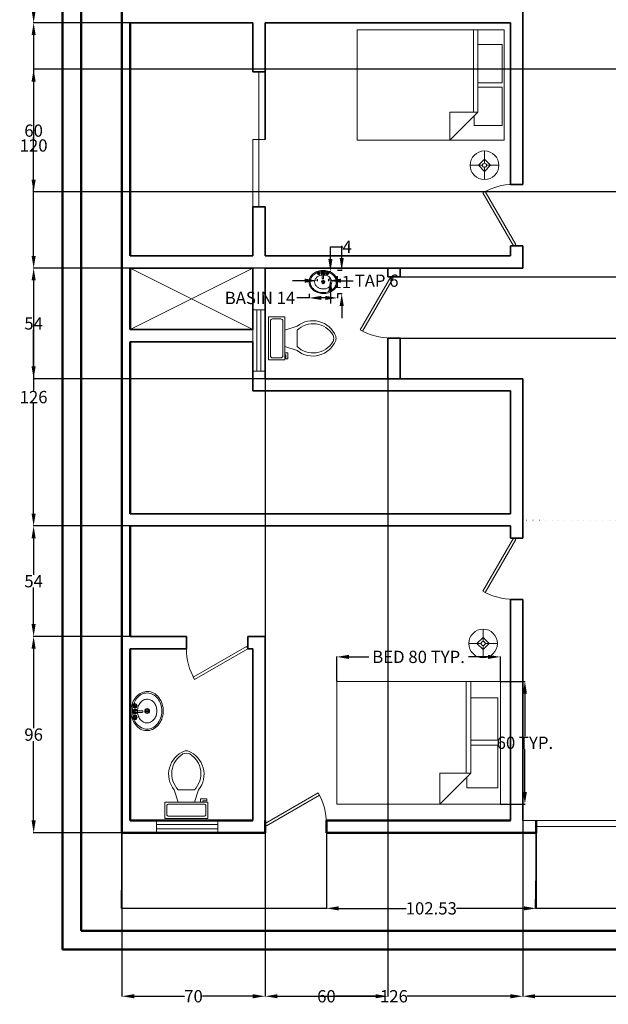
# Model space of a CAD drawing. Units: inches. Extents: x 910 to 1553, y 598 to 1516.
# Tile 1 of 6: x 910 to 1198, y 598 to 1079. Entities that reach past the tile are written whole.
import ezdxf

# ---------------------------------------------------------------- set-up
doc = ezdxf.new("R2010")
doc.units = ezdxf.units.IN
doc.header["$MEASUREMENT"] = 0
doc.linetypes.add('ACAD_ISO07W100', pattern=[3, 0, -3])
for name, color, linetype, lineweight in [('A-ANNO-DIMS', 2, 'Continuous', 18), ('A-FLOR-BALC', 8, 'Continuous', 25), ('A-FLOR-OPEN', 8, 'Continuous', 13), ('A-FLOR-OVHD', 8, 'ACAD_ISO07W100', 13), ('doors', 2, 'Continuous', 18), ('furniture', 11, 'Continuous', 18), ('Inner wall', 230, 'Continuous', 35), ('outer wall', 231, 'Continuous', 50), ('sanitory', 141, 'Continuous', 18), ('windows', 6, 'Continuous', 18)]:
    doc.layers.add(name, color=color, linetype=linetype, lineweight=lineweight)
doc.styles.get("Standard").update_dxf_attribs({"font": 'arial.ttf'})
doc.dimstyles.get("Standard").update_dxf_attribs({"dimtxt": 6, "dimasz": 6, "dimexe": 0.18, "dimexo": 0.0625, "dimgap": 0.09, "dimtad": 0, "dimtih": 1, "dimtoh": 1, "dimdec": 0, "dimzin": 0, "dimdsep": 46, "dimlunit": 3, "dimtxsty": 'Standard', "dimcen": 0.09, "dimadec": 0, "dimazin": 0, "dimtfac": 1, "dimtdec": 0, "dimtofl": 0, "dimtmove": 0, "dimatfit": 3, "dimfxl": 1, "dimtolj": 1, "dimtzin": 0, "dimarcsym": 0})

# ---------------------------------------------------------------- blocks, each defined once
blk = doc.blocks.new('*U7')
for p, q in [((-40, 0), (-40, 6)), ((0, 0), (0, 6))]:
    blk.add_line(p, q)
blk.add_lwpolyline([(0, 0), (-34.64, -20), (-35.52, -18.48), (-0.88, 1.52)], close=True)
blk.add_arc((0, 0), 40, 180, 210)
blk = doc.blocks.new('*U2')
for p, q in [((0, 0), (0, -6)), ((40, 0), (40, -6))]:
    blk.add_line(p, q)
blk.add_lwpolyline([(0, 0), (34.64, 20), (35.52, 18.48), (0.87, -1.52)], close=True)
blk.add_arc((0, 0), 40, 0, 30)
blk = doc.blocks.new('*U5')
for p, q in [((0, 0), (0, -6)), ((-40, 0), (-40, -6))]:
    blk.add_line(p, q)
blk.add_lwpolyline([(0, 0), (-34.64, 20), (-35.52, 18.48), (-0.88, -1.52)], close=True)
blk.add_arc((0, 0), 40, 150, 180)
blk = doc.blocks.new('Toilet - top')
for p, q in [((9.5, -6), (9.5, -2)), ((-10, -8.5), (-8, -8.5)), ((-10, -9.5), (-10, -8.5)), ((-7, -9.5), (-10, -9.5)), ((-8, -8.5), (-8, -8)), ((-7, -8), (-7, -9.5)), ((-4, -8), (-6, -14)), ((4, -8), (6, -14)), ((4, -14), (-4, -14))]:
    blk.add_line(p, q)
blk.add_lwpolyline([(10.5, -8), (10.5, 0), (-10.5, 0), (-10.5, -8)], close=True)
for points in [[(-9.5, -2), (-9.5, -6)], [(8.5, -1), (-8.5, -1)], [(-8.5, -7), (8.5, -7)]]:
    blk.add_lwpolyline(points)
for centre, radius, start, end in [((-8.62, -1.88), 0.884, 81.8699, 188.1301), ((8.62, -1.88), 0.884, 351.8699, 98.1301), ((-8.62, -6.12), 0.884, 171.8699, 278.1301), ((8.62, -6.12), 0.884, 261.8699, 8.1301), ((3.52, -21.58), 12.17, 141.4691, 247.9714), ((4.2, -21.82), 11.33, 136.3677, 238.9468), ((-3.52, -21.58), 12.17, 292.0284, 38.5307), ((-4.2, -21.82), 11.33, 301.053, 43.6321), ((0, -27.88), 4, 245.7318, 294.2682), ((0, -29), 4, 254.8605, 285.1395)]:
    blk.add_arc(centre, radius, start, end)
blk = doc.blocks.new('Bed - Queen')
for p, q in [((0, -80.00003), (0, 0)), ((0, 0), (59.99999, 0)), ((59.99999, 0), (59.99999, -80.00003)), ((7.99999, -1.2), (28.79998, -1.2)), ((7.99999, -14.4), (7.99999, -1.2)), ((28.79998, -1.2), (28.79998, -14.4)), ((31.19999, -1.2), (51.99999, -1.2)), ((31.19999, -14.4), (31.19999, -1.2)), ((51.99999, -1.2), (51.99999, -16.4)), ((0, -14.4), (44.8, -14.4)), ((59.99999, -29.6), (44.8, -14.4)), ((44.8, -14.4), (44.8, -29.6)), ((44.8, -16.8), (0, -16.8)), ((51.99999, -16.4), (46.79936, -16.4)), ((44.8, -29.6), (59.99999, -29.6)), ((59.99999, -80.00003), (0, -80.00003))]:
    blk.add_line(p, q)
blk = doc.blocks.new('Lamp - Table')
for p, q in [((0, 7), (0, 1)), ((-1, 0), (-7, 0)), ((0, 3), (-3, 0)), ((-3, 0), (0, -3)), ((3, 0), (0, 3)), ((0, -3), (3, 0)), ((1, 0), (7, 0)), ((0, -1), (0, -7))]:
    blk.add_line(p, q)
for radius in [7, 1]:
    blk.add_circle((0, 0), radius)
blk = doc.blocks.new('Faucet - Bathroom top')
for p, q in [((-4.107, 0.125), (-4.375, 0.125)), ((-3.75, 0.4788), (-3.75, 0.75)), ((-3.5, 0.482), (-3.5, 0.75)), ((-3.1461, 0.125), (-2.875, 0.125)), ((3.143, 0.125), (2.875, 0.125)), ((3.5, 0.4788), (3.5, 0.75)), ((3.75, 0.482), (3.75, 0.75)), ((4.1039, 0.125), (4.375, 0.125)), ((-4.1039, -0.125), (-4.375, -0.125)), ((-3.75, -0.4821), (-3.75, -0.75)), ((-3.5, -0.4789), (-3.5, -0.75)), ((-3.143, -0.125), (-2.875, -0.125)), ((-0.5, -0.8639), (-0.5, -4.5)), ((0.5, -4.5), (0.5, -0.8631)), ((3.1461, -0.125), (2.875, -0.125)), ((3.5, -0.4821), (3.5, -0.75)), ((3.75, -0.4789), (3.75, -0.75)), ((4.107, -0.125), (4.375, -0.125))]:
    blk.add_line(p, q)
for centre, radius in [((-3.625, 0), 1.375), ((-4.625, 0), 0.2795), ((-3.625, 0), 0.5), ((-3.625, 1), 0.2795), ((-2.625, 0), 0.2795), ((0, 0), 0.5), ((3.625, 0), 1.375), ((2.625, 0), 0.2795), ((3.625, 0), 0.5), ((3.625, 1), 0.2795), ((4.625, 0), 0.2795), ((-3.625, -1), 0.2795), ((3.625, -1), 0.2795)]:
    blk.add_circle(centre, radius)
for centre, radius, start, end in [((-3.625, 0), 1, 105.2407, 164.2093), ((-3.625, 0), 1, 16.44125, 74.07887), ((0, 0), 1.5, 289.6514, 250.3603), ((0, 0), 1, 300.3431, 239.7554), ((3.625, 0), 1, 106.12, 164.0884), ((3.625, 0), 1, 16.23422, 73.90469), ((-3.625, 0), 1, 196.2342, 253.9047), ((-3.625, 0), 1, 286.12, 344.0884), ((0, -4.5), 0.5, 180, 0), ((3.625, 0), 1, 196.4413, 254.0789), ((3.625, 0), 1, 285.2407, 344.2093)]:
    blk.add_arc(centre, radius, start, end)
blk = doc.blocks.new('Sink - Oval top')
for p, q in [((-1, 0), (1, 0)), ((0, 1), (0, -1))]:
    blk.add_line(p, q)
for points in [[(-12.23, 0.39, 0.117634), (-11.46, -3.36, 0.104469), (-8.88, -6.8, 0.090016), (-5.08, -9.07, 0.08192), (-0.32, -10.02, 0.08192), (4.49, -9.38, 0.090016), (8.42, -7.36, 0.104469), (11.22, -4.09, 0.117634), (12.23, -0.39, 0.117634), (11.46, 3.36, 0.104469), (8.88, 6.8, 0.090016), (5.08, 9.07, 0.08192), (0.32, 10.02, 0.08192), (-4.49, 9.38, 0.090016), (-8.42, 7.36, 0.104469), (-11.22, 4.09, 0.117634)], [(-11.29, 0.16, 0.118622), (-10.52, -3.25, 0.104678), (-8.07, -6.36, 0.089562), (-4.54, -8.37, 0.081185), (-0.13, -9.15, 0.081185), (4.3, -8.49, 0.089562), (7.89, -6.58, 0.104678), (10.42, -3.55, 0.118622), (11.29, -0.16, 0.118622), (10.52, 3.25, 0.104678), (8.07, 6.36, 0.089562), (4.54, 8.37, 0.081185), (0.13, 9.15, 0.081185), (-4.3, 8.49, 0.089562), (-7.89, 6.58, 0.104678), (-10.42, 3.55, 0.118622)], [(-7.42, 0.08, 0.118283), (-6.91, -2.17, 0.104607), (-5.29, -4.21, 0.089718), (-2.97, -5.53, 0.081436), (-0.07, -6.04, 0.081436), (2.84, -5.59, 0.089718), (5.2, -4.33, 0.104607), (6.86, -2.32, 0.118283), (7.42, -0.08, 0.118283), (6.91, 2.17, 0.104607), (5.29, 4.21, 0.089718), (2.97, 5.53, 0.081436), (0.07, 6.04, 0.081436), (-2.84, 5.59, 0.089718), (-5.2, 4.33, 0.104607), (-6.86, 2.32, 0.118283)]]:
    blk.add_lwpolyline(points, format="xyb", close=True)
for radius in [1.5, 1]:
    blk.add_circle((0, 0), radius)
blk = doc.blocks.new('WIN-30X6')
for p, q in [((0, 6), (30, 6)), ((0, 0), (0, 6)), ((30, 6), (30, 0)), ((0, 4), (30, 4)), ((30, 2), (0, 2)), ((30, 0), (0, 0))]:
    blk.add_line(p, q)
blk = doc.blocks.new('VERANDA-EDGE-DEEP')
for p, q in [((0.23, 17.99), (0.23, 36.98)), ((100.23, 36.98), (100.23, 17.99)), ((0, 0), (0.23, 17.99)), ((100.23, 17.99), (100.23, 0)), ((100.23, 0), (0, 0))]:
    blk.add_line(p, q)
blk = doc.blocks.new('*D25')
at = {"layer": 'A-ANNO-DIMS', "color": 0, "lineweight": -2, "transparency": 16777216}
for p, q in [((1064.74, 756.03), (1064.74, 768.14)), ((1070.74, 767.96), (1080.4, 767.96)), ((1138.74, 767.96), (1129.09, 767.96)), ((1144.74, 756.03), (1144.74, 768.14))]:
    blk.add_line(p, q, dxfattribs=at)
for points in [[(1070.74, 768.96), (1070.74, 766.96), (1064.74, 767.96)], [(1138.74, 768.96), (1138.74, 766.96), (1144.74, 767.96)]]:
    blk.add_solid(points, dxfattribs=at)
at = {"layer": 'Defpoints', "color": 0, "lineweight": -2, "transparency": 16777216}
for p in [(1144.74, 767.96), (1064.74, 755.96), (1144.74, 755.96)]:
    blk.add_point(p, dxfattribs=at)
at = {"layer": 'A-ANNO-DIMS', "color": 0, "transparency": 16777216, "insert": (1104.74, 767.96), "char_height": 6, "attachment_point": 5}
blk.add_mtext('\\A1;BED 80 TYP.', dxfattribs=at)
blk = doc.blocks.new('*D26')
at = {"layer": 'A-ANNO-DIMS', "color": 0, "lineweight": -2, "transparency": 16777216}
for p, q in [((1144.81, 755.96), (1156.92, 755.96)), ((1156.74, 749.96), (1156.74, 729.12)), ((1156.74, 701.96), (1156.74, 722.81)), ((1144.81, 695.96), (1156.92, 695.96))]:
    blk.add_line(p, q, dxfattribs=at)
for points in [[(1155.74, 749.96), (1157.74, 749.96), (1156.74, 755.96)], [(1155.74, 701.96), (1157.74, 701.96), (1156.74, 695.96)]]:
    blk.add_solid(points, dxfattribs=at)
at = {"layer": 'Defpoints', "color": 0, "lineweight": -2, "transparency": 16777216}
for p in [(1144.74, 755.96), (1144.74, 695.96), (1156.74, 695.96)]:
    blk.add_point(p, dxfattribs=at)
at = {"layer": 'A-ANNO-DIMS', "color": 0, "transparency": 16777216, "insert": (1156.74, 725.96), "char_height": 6, "attachment_point": 5}
blk.add_mtext('\\A1;60 TYP.', dxfattribs=at)
blk = doc.blocks.new('*D33')
at = {"layer": 'A-ANNO-DIMS', "color": 0, "lineweight": -2, "transparency": 16777216}
for p, q in [((1051.19, 945.48), (1051.19, 943.27)), ((1065.09, 945.48), (1065.09, 943.27)), ((1051.19, 943.45), (1045.19, 943.45)), ((1059.09, 943.45), (1057.19, 943.45))]:
    blk.add_line(p, q, dxfattribs=at)
for points in [[(1057.19, 944.45), (1057.19, 942.45), (1051.19, 943.45)], [(1059.09, 944.45), (1059.09, 942.45), (1065.09, 943.45)]]:
    blk.add_solid(points, dxfattribs=at)
at = {"layer": 'Defpoints', "color": 0, "lineweight": -2, "transparency": 16777216}
for p in [(1051.19, 945.54), (1065.09, 945.54), (1051.19, 943.45)]:
    blk.add_point(p, dxfattribs=at)
at = {"layer": 'A-ANNO-DIMS', "color": 0, "transparency": 16777216, "insert": (1027.2, 943.45), "char_height": 6, "attachment_point": 5}
blk.add_mtext('\\A1;BASIN 14', dxfattribs=at)
blk = doc.blocks.new('*D34')
at = {"layer": 'A-ANNO-DIMS', "color": 0, "lineweight": -2, "transparency": 16777216}
for p, q in [((1067.17, 962.94), (1067.17, 968.94)), ((1065.15, 956.94), (1067.35, 956.94)), ((1065.15, 945.54), (1067.35, 945.54)), ((1067.17, 939.54), (1067.17, 933.54))]:
    blk.add_line(p, q, dxfattribs=at)
for points in [[(1066.17, 962.94), (1068.17, 962.94), (1067.17, 956.94)], [(1066.17, 939.54), (1068.17, 939.54), (1067.17, 945.54)]]:
    blk.add_solid(points, dxfattribs=at)
at = {"layer": 'Defpoints', "color": 0, "lineweight": -2, "transparency": 16777216}
for p in [(1065.09, 956.94), (1065.09, 945.54), (1067.17, 945.54)]:
    blk.add_point(p, dxfattribs=at)
at = {"layer": 'A-ANNO-DIMS', "color": 0, "transparency": 16777216, "insert": (1067.17, 951.24), "char_height": 6, "attachment_point": 5}
blk.add_mtext('\\A1;11', dxfattribs=at)
blk = doc.blocks.new('*D37')
at = {"layer": 'A-ANNO-DIMS', "color": 0, "lineweight": -2, "transparency": 16777216}
for p, q in [((1049.13, 951.87), (1043.13, 951.87)), ((1055.13, 952.66), (1055.13, 951.69)), ((1060.79, 952.66), (1060.79, 951.69)), ((1066.79, 951.87), (1072.79, 951.87))]:
    blk.add_line(p, q, dxfattribs=at)
for points in [[(1049.13, 952.87), (1049.13, 950.87), (1055.13, 951.87)], [(1066.79, 952.87), (1066.79, 950.87), (1060.79, 951.87)]]:
    blk.add_solid(points, dxfattribs=at)
at = {"layer": 'Defpoints', "color": 0, "lineweight": -2, "transparency": 16777216}
for p in [(1055.13, 952.72), (1060.79, 952.72), (1060.79, 951.87)]:
    blk.add_point(p, dxfattribs=at)
at = {"layer": 'A-ANNO-DIMS', "color": 0, "transparency": 16777216, "insert": (1084.24, 951.87), "char_height": 6, "attachment_point": 5}
blk.add_mtext('\\A1;TAP 6', dxfattribs=at)
blk = doc.blocks.new('*D38')
at = {"layer": 'A-ANNO-DIMS', "color": 0, "lineweight": -2, "transparency": 16777216}
for p, q in [((1061.64, 962.4), (1061.64, 968.4)), ((1061.64, 968.4), (1067.64, 968.4)), ((1060.85, 956.4), (1061.82, 956.4)), ((1060.85, 952.72), (1061.82, 952.72)), ((1061.64, 946.72), (1061.64, 940.72))]:
    blk.add_line(p, q, dxfattribs=at)
for points in [[(1060.64, 962.4), (1062.64, 962.4), (1061.64, 956.4)], [(1060.64, 946.72), (1062.64, 946.72), (1061.64, 952.72)]]:
    blk.add_solid(points, dxfattribs=at)
at = {"layer": 'Defpoints', "color": 0, "lineweight": -2, "transparency": 16777216}
for p in [(1060.79, 956.4), (1061.64, 956.4), (1060.79, 952.72)]:
    blk.add_point(p, dxfattribs=at)
at = {"layer": 'A-ANNO-DIMS', "color": 0, "transparency": 16777216, "insert": (1069.81, 968.4), "char_height": 6, "attachment_point": 5}
blk.add_mtext('\\A1;4', dxfattribs=at)
blk = doc.blocks.new('*D57')
at = {"layer": 'A-ANNO-DIMS', "color": 0, "lineweight": -2, "transparency": 16777216}
for p, q in [((959.7, 681.91), (959.7, 601.86)), ((1029.7, 681.91), (1029.7, 601.86)), ((965.7, 602.04), (990.35, 602.04)), ((1023.7, 602.04), (999.05, 602.04))]:
    blk.add_line(p, q, dxfattribs=at)
for points in [[(965.7, 603.04), (965.7, 601.04), (959.7, 602.04)], [(1023.7, 603.04), (1023.7, 601.04), (1029.7, 602.04)]]:
    blk.add_solid(points, dxfattribs=at)
at = {"layer": 'Defpoints', "color": 0, "lineweight": -2, "transparency": 16777216}
for p in [(959.7, 681.97), (1029.7, 681.97), (1029.7, 602.04)]:
    blk.add_point(p, dxfattribs=at)
at = {"layer": 'A-ANNO-DIMS', "color": 0, "transparency": 16777216, "insert": (994.7, 602.04), "char_height": 6, "attachment_point": 5}
blk.add_mtext('\\A1;70', dxfattribs=at)
blk = doc.blocks.new('*D58')
at = {"layer": 'A-ANNO-DIMS', "color": 0, "lineweight": -2, "transparency": 16777216}
for p, q in [((1155.7, 687.91), (1155.7, 601.86)), ((1029.7, 681.91), (1029.7, 601.86)), ((1035.7, 602.04), (1086.27, 602.04)), ((1149.7, 602.04), (1099.13, 602.04))]:
    blk.add_line(p, q, dxfattribs=at)
for points in [[(1035.7, 603.04), (1035.7, 601.04), (1029.7, 602.04)], [(1149.7, 603.04), (1149.7, 601.04), (1155.7, 602.04)]]:
    blk.add_solid(points, dxfattribs=at)
at = {"layer": 'Defpoints', "color": 0, "lineweight": -2, "transparency": 16777216}
for p in [(1155.7, 687.97), (1029.7, 681.97), (1155.7, 602.04)]:
    blk.add_point(p, dxfattribs=at)
at = {"layer": 'A-ANNO-DIMS', "color": 0, "transparency": 16777216, "insert": (1092.7, 602.04), "char_height": 6, "attachment_point": 5}
blk.add_mtext('\\A1;126', dxfattribs=at)
blk = doc.blocks.new('*D59')
at = {"layer": 'A-ANNO-DIMS', "color": 0, "lineweight": -2, "transparency": 16777216}
for p, q in [((1155.7, 687.91), (1155.7, 601.86)), ((1281.7, 687.91), (1281.7, 601.86)), ((1161.7, 602.04), (1212.27, 602.04)), ((1275.7, 602.04), (1225.13, 602.04))]:
    blk.add_line(p, q, dxfattribs=at)
for points in [[(1161.7, 603.04), (1161.7, 601.04), (1155.7, 602.04)], [(1275.7, 603.04), (1275.7, 601.04), (1281.7, 602.04)]]:
    blk.add_solid(points, dxfattribs=at)
at = {"layer": 'Defpoints', "color": 0, "lineweight": -2, "transparency": 16777216}
for p in [(1155.7, 687.97), (1281.7, 687.97), (1281.7, 602.04)]:
    blk.add_point(p, dxfattribs=at)
at = {"layer": 'A-ANNO-DIMS', "color": 0, "transparency": 16777216, "insert": (1218.7, 602.04), "char_height": 6, "attachment_point": 5}
blk.add_mtext('\\A1;126', dxfattribs=at)
blk = doc.blocks.new('*D62')
at = {"layer": 'A-ANNO-DIMS', "color": 0, "lineweight": -2, "transparency": 16777216}
for p, q in [((963.64, 777.97), (916.34, 777.97)), ((916.52, 771.97), (916.52, 733.12)), ((916.52, 687.97), (916.52, 726.82)), ((959.64, 681.97), (916.34, 681.97))]:
    blk.add_line(p, q, dxfattribs=at)
for points in [[(915.52, 771.97), (917.52, 771.97), (916.52, 777.97)], [(915.52, 687.97), (917.52, 687.97), (916.52, 681.97)]]:
    blk.add_solid(points, dxfattribs=at)
at = {"layer": 'Defpoints', "color": 0, "lineweight": -2, "transparency": 16777216}
for p in [(916.52, 777.97), (963.7, 777.97), (959.7, 681.97)]:
    blk.add_point(p, dxfattribs=at)
at = {"layer": 'A-ANNO-DIMS', "color": 0, "transparency": 16777216, "insert": (916.52, 729.97), "char_height": 6, "attachment_point": 5}
blk.add_mtext('\\A1;96', dxfattribs=at)
blk = doc.blocks.new('*D63')
at = {"layer": 'A-ANNO-DIMS', "color": 0, "lineweight": -2, "transparency": 16777216}
for p, q in [((963.64, 831.97), (916.34, 831.97)), ((916.52, 825.97), (916.52, 808.11)), ((916.52, 783.97), (916.52, 801.83)), ((963.64, 777.97), (916.34, 777.97))]:
    blk.add_line(p, q, dxfattribs=at)
for points in [[(915.52, 825.97), (917.52, 825.97), (916.52, 831.97)], [(915.52, 783.97), (917.52, 783.97), (916.52, 777.97)]]:
    blk.add_solid(points, dxfattribs=at)
at = {"layer": 'Defpoints', "color": 0, "lineweight": -2, "transparency": 16777216}
for p in [(916.52, 831.97), (963.7, 831.97), (963.7, 777.97)]:
    blk.add_point(p, dxfattribs=at)
at = {"layer": 'A-ANNO-DIMS', "color": 0, "transparency": 16777216, "insert": (916.52, 804.97), "char_height": 6, "attachment_point": 5}
blk.add_mtext('\\A1;54', dxfattribs=at)
blk = doc.blocks.new('*D64')
at = {"layer": 'A-ANNO-DIMS', "color": 0, "lineweight": -2, "transparency": 16777216}
for p, q in [((963.64, 957.97), (916.34, 957.97)), ((916.52, 951.97), (916.52, 898.12)), ((916.52, 837.97), (916.52, 891.82)), ((963.64, 831.97), (916.34, 831.97))]:
    blk.add_line(p, q, dxfattribs=at)
for points in [[(915.52, 951.97), (917.52, 951.97), (916.52, 957.97)], [(915.52, 837.97), (917.52, 837.97), (916.52, 831.97)]]:
    blk.add_solid(points, dxfattribs=at)
at = {"layer": 'Defpoints', "color": 0, "lineweight": -2, "transparency": 16777216}
for p in [(916.52, 957.97), (963.7, 957.97), (963.7, 831.97)]:
    blk.add_point(p, dxfattribs=at)
at = {"layer": 'A-ANNO-DIMS', "color": 0, "transparency": 16777216, "insert": (916.52, 894.97), "char_height": 6, "attachment_point": 5}
blk.add_mtext('\\A1;126', dxfattribs=at)
blk = doc.blocks.new('*D65')
at = {"layer": 'A-ANNO-DIMS', "color": 0, "lineweight": -2, "transparency": 16777216}
for p, q in [((963.64, 1077.97), (916.34, 1077.97)), ((916.52, 1071.97), (916.52, 1021.12)), ((916.52, 963.97), (916.52, 1014.82)), ((963.64, 957.97), (916.34, 957.97))]:
    blk.add_line(p, q, dxfattribs=at)
for points in [[(915.52, 1071.97), (917.52, 1071.97), (916.52, 1077.97)], [(915.52, 963.97), (917.52, 963.97), (916.52, 957.97)]]:
    blk.add_solid(points, dxfattribs=at)
at = {"layer": 'Defpoints', "color": 0, "lineweight": -2, "transparency": 16777216}
for p in [(916.52, 1077.97), (963.7, 1077.97), (963.7, 957.97)]:
    blk.add_point(p, dxfattribs=at)
at = {"layer": 'A-ANNO-DIMS', "color": 0, "transparency": 16777216, "insert": (916.52, 1017.97), "char_height": 6, "attachment_point": 5}
blk.add_mtext('\\A1;120', dxfattribs=at)
blk = doc.blocks.new('*D66')
at = {"layer": 'A-ANNO-DIMS', "color": 0, "lineweight": -2, "transparency": 16777216}
for p, q in [((963.64, 1179.97), (916.34, 1179.97)), ((916.52, 1173.97), (916.52, 1132.12)), ((916.52, 1083.97), (916.52, 1125.82)), ((963.64, 1077.97), (916.34, 1077.97))]:
    blk.add_line(p, q, dxfattribs=at)
for points in [[(915.52, 1173.97), (917.52, 1173.97), (916.52, 1179.97)], [(915.52, 1083.97), (917.52, 1083.97), (916.52, 1077.97)]]:
    blk.add_solid(points, dxfattribs=at)
at = {"layer": 'Defpoints', "color": 0, "lineweight": -2, "transparency": 16777216}
for p in [(916.52, 1179.97), (963.7, 1179.97), (963.7, 1077.97)]:
    blk.add_point(p, dxfattribs=at)
at = {"layer": 'A-ANNO-DIMS', "color": 0, "transparency": 16777216, "insert": (916.52, 1128.97), "char_height": 6, "attachment_point": 5}
blk.add_mtext('\\A1;102', dxfattribs=at)
blk = doc.blocks.new('*D74')
at = {"layer": 'A-ANNO-DIMS', "color": 0, "lineweight": -2, "transparency": 16777216}
for p, q in [((1029.7, 903.91), (1029.7, 601.86)), ((1089.7, 903.91), (1089.7, 601.86)), ((1035.7, 602.04), (1055.31, 602.04)), ((1083.7, 602.04), (1064.09, 602.04))]:
    blk.add_line(p, q, dxfattribs=at)
for points in [[(1035.7, 603.04), (1035.7, 601.04), (1029.7, 602.04)], [(1083.7, 603.04), (1083.7, 601.04), (1089.7, 602.04)]]:
    blk.add_solid(points, dxfattribs=at)
at = {"layer": 'Defpoints', "color": 0, "lineweight": -2, "transparency": 16777216}
for p in [(1029.7, 903.97), (1089.7, 903.97), (1089.7, 602.04)]:
    blk.add_point(p, dxfattribs=at)
at = {"layer": 'A-ANNO-DIMS', "color": 0, "transparency": 16777216, "insert": (1059.7, 602.04), "char_height": 6, "attachment_point": 5}
blk.add_mtext('\\A1;60', dxfattribs=at)
blk = doc.blocks.new('*D75')
at = {"layer": 'A-ANNO-DIMS', "color": 0, "lineweight": -2, "transparency": 16777216}
for p, q in [((1029.64, 957.97), (916.34, 957.97)), ((916.52, 951.97), (916.52, 934.11)), ((916.52, 909.97), (916.52, 927.83)), ((1029.64, 903.97), (916.34, 903.97))]:
    blk.add_line(p, q, dxfattribs=at)
for points in [[(915.52, 951.97), (917.52, 951.97), (916.52, 957.97)], [(915.52, 909.97), (917.52, 909.97), (916.52, 903.97)]]:
    blk.add_solid(points, dxfattribs=at)
at = {"layer": 'Defpoints', "color": 0, "lineweight": -2, "transparency": 16777216}
for p in [(916.52, 957.97), (1029.7, 957.97), (1029.7, 903.97)]:
    blk.add_point(p, dxfattribs=at)
at = {"layer": 'A-ANNO-DIMS', "color": 0, "transparency": 16777216, "insert": (916.52, 930.97), "char_height": 6, "attachment_point": 5}
blk.add_mtext('\\A1;54', dxfattribs=at)
blk = doc.blocks.new('*D76')
at = {"layer": 'A-ANNO-DIMS', "color": 0, "lineweight": -2, "transparency": 16777216}
for p, q in [((1089.76, 953.83), (1544.83, 953.83)), ((1544.65, 947.83), (1544.65, 941.98)), ((1544.65, 929.83), (1544.65, 935.67)), ((1089.76, 923.83), (1544.83, 923.83))]:
    blk.add_line(p, q, dxfattribs=at)
for points in [[(1543.65, 947.83), (1545.65, 947.83), (1544.65, 953.83)], [(1543.65, 929.83), (1545.65, 929.83), (1544.65, 923.83)]]:
    blk.add_solid(points, dxfattribs=at)
at = {"layer": 'Defpoints', "color": 0, "lineweight": -2, "transparency": 16777216}
for p in [(1089.7, 953.83), (1544.65, 953.83), (1089.7, 923.83)]:
    blk.add_point(p, dxfattribs=at)
at = {"layer": 'A-ANNO-DIMS', "color": 0, "transparency": 16777216, "insert": (1544.65, 938.83), "char_height": 6, "attachment_point": 5}
blk.add_mtext('\\A1;30', dxfattribs=at)
blk = doc.blocks.new('*D85')
at = {"layer": 'A-ANNO-DIMS', "color": 0, "lineweight": -2, "transparency": 16777216}
for p, q in [((1287.64, 1055.24), (916.34, 1055.24)), ((916.52, 1049.24), (916.52, 1028.4)), ((916.52, 1001.24), (916.52, 1022.09)), ((1287.64, 995.24), (916.34, 995.24))]:
    blk.add_line(p, q, dxfattribs=at)
for points in [[(915.52, 1049.24), (917.52, 1049.24), (916.52, 1055.24)], [(915.52, 1001.24), (917.52, 1001.24), (916.52, 995.24)]]:
    blk.add_solid(points, dxfattribs=at)
at = {"layer": 'Defpoints', "color": 0, "lineweight": -2, "transparency": 16777216}
for p in [(916.52, 1055.24), (1287.7, 1055.24), (1287.7, 995.24)]:
    blk.add_point(p, dxfattribs=at)
at = {"layer": 'A-ANNO-DIMS', "color": 0, "transparency": 16777216, "insert": (916.52, 1025.24), "char_height": 6, "attachment_point": 5}
blk.add_mtext('\\A1;60', dxfattribs=at)
blk = doc.blocks.new('*D87')
at = {"layer": 'A-ANNO-DIMS', "color": 0, "lineweight": -2, "transparency": 16777216}
for p, q in [((1059.7, 687.91), (1059.7, 644.84)), ((1162.23, 687.91), (1162.23, 644.84)), ((1065.7, 645.02), (1098.71, 645.02)), ((1156.23, 645.02), (1123.23, 645.02))]:
    blk.add_line(p, q, dxfattribs=at)
for points in [[(1065.7, 646.02), (1065.7, 644.02), (1059.7, 645.02)], [(1156.23, 646.02), (1156.23, 644.02), (1162.23, 645.02)]]:
    blk.add_solid(points, dxfattribs=at)
at = {"layer": 'Defpoints', "color": 0, "lineweight": -2, "transparency": 16777216}
for p in [(1059.7, 687.97), (1162.23, 687.97), (1059.7, 645.02)]:
    blk.add_point(p, dxfattribs=at)
at = {"layer": 'A-ANNO-DIMS', "color": 0, "transparency": 16777216, "insert": (1110.97, 645.02), "char_height": 6, "attachment_point": 5}
blk.add_mtext('\\A1;102.53', dxfattribs=at)

msp = doc.modelspace()

# ---------------------------------------------------------------- linework, layer by layer
at = {"layer": 'A-FLOR-BALC'}
for p, q in [((1162.234, 662.984), (1162.234, 687.969)), ((1162.004, 644.993), (1162.234, 662.984)), ((1262.234, 644.993), (1162.004, 644.993))]:
    msp.add_line(p, q, dxfattribs=at)
at = {"layer": 'A-FLOR-OPEN'}
for p, q in [((963.7, 957.969), (1023.7, 927.969)), ((1023.7, 957.969), (963.7, 927.969))]:
    msp.add_line(p, q, dxfattribs=at)
at = {"layer": 'A-FLOR-OVHD'}
msp.add_line((1281.7, 834.815), (1155.7, 834.815), dxfattribs=at)
at = {"layer": 'doors'}
for p, q in [((1026.7, 1053.969), (1026.7, 987.969)), ((1026.7, 1053.969), (1029.7, 1053.969)), ((1029.7, 1020.969), (1029.7, 1053.969)), ((1029.7, 1020.969), (1023.7, 1020.969)), ((1023.7, 1020.969), (1023.7, 963.969)), ((1023.7, 987.969), (1026.7, 987.969)), ((1155.7, 687.969), (1212.234, 687.969)), ((1162.234, 687.969), (1162.234, 684.969)), ((1162.234, 684.969), (1262.234, 684.969))]:
    msp.add_line(p, q, dxfattribs=at)
at = {"layer": 'Inner wall'}
for p, q in [((1155.7, 1145.953), (1155.7, 998.911)), ((1023.7, 1077.969), (963.7, 1077.969)), ((1023.7, 1077.969), (1023.7, 1053.969)), ((1149.7, 1077.969), (1029.7, 1077.969)), ((1029.7, 1077.969), (1029.7, 1020.969)), ((1149.7, 1077.969), (1149.7, 998.911)), ((1029.7, 1053.969), (1023.7, 1053.969)), ((1023.7, 987.969), (1029.7, 987.969)), ((1023.7, 963.969), (1023.7, 987.969)), ((1029.7, 987.969), (1029.7, 963.969)), ((1149.7, 968.911), (1149.7, 963.969)), ((1155.7, 968.911), (1155.7, 963.969)), ((1155.7, 968.911), (1155.7, 957.969)), ((963.7, 963.969), (1023.7, 963.969)), ((1029.7, 963.969), (1149.7, 963.969)), ((963.7, 957.969), (1023.7, 957.969)), ((1023.7, 957.969), (1023.7, 927.969)), ((1029.7, 957.969), (1155.7, 957.969)), ((1029.7, 957.969), (1029.7, 903.969)), ((1089.7, 957.969), (1089.7, 953.828)), ((1095.7, 957.969), (1095.7, 953.828)), ((1023.7, 927.969), (963.7, 927.969)), ((1023.7, 921.969), (963.7, 921.969)), ((1023.7, 921.969), (1023.7, 897.969)), ((1089.7, 923.828), (1089.7, 903.969)), ((1095.7, 923.828), (1095.7, 903.969)), ((1029.7, 903.969), (1155.7, 903.969)), ((1155.7, 903.969), (1155.7, 826.061)), ((1023.7, 897.969), (1149.7, 897.969)), ((1149.7, 897.969), (1149.7, 837.969)), ((963.7, 837.969), (1149.7, 837.969)), ((963.7, 831.969), (1149.7, 831.969)), ((1149.7, 831.969), (1149.7, 826.061)), ((1155.7, 831.969), (1155.7, 826.061)), ((1149.7, 796.061), (1149.7, 687.969)), ((1155.7, 796.061), (1155.7, 687.969)), ((963.7, 777.969), (991.209, 777.969)), ((1021.209, 777.969), (1029.7, 777.969)), ((1029.7, 777.969), (1029.7, 687.969)), ((963.7, 771.969), (991.209, 771.969)), ((1021.209, 771.969), (1023.7, 771.969)), ((1023.7, 771.969), (1023.7, 687.969))]:
    msp.add_line(p, q, dxfattribs=at)
for points in [[(1149.7, 998.911), (1155.7, 998.911)], [(1155.7, 968.911), (1149.7, 968.911)], [(1089.7, 953.828), (1095.7, 953.828)], [(1095.7, 923.828), (1089.7, 923.828)], [(1149.7, 826.061), (1155.7, 826.061)], [(1155.7, 796.061), (1149.7, 796.061)], [(991.209, 771.969), (991.209, 777.969)], [(1021.209, 777.969), (1021.209, 771.969)]]:
    msp.add_lwpolyline(points, dxfattribs=at)
at = {"layer": 'outer wall'}
for p, q in [((939.7, 1479.969), (939.7, 633.969)), ((959.7, 1449.969), (959.7, 681.969)), ((963.7, 1077.969), (963.7, 963.969)), ((963.7, 957.969), (963.7, 927.969)), ((963.7, 921.969), (963.7, 837.969)), ((963.7, 831.969), (963.7, 777.969)), ((963.7, 771.969), (963.7, 687.969)), ((963.7, 687.969), (1023.7, 687.969)), ((1059.7, 687.969), (1149.7, 687.969)), ((1162.234, 681.969), (1162.234, 687.969)), ((963.7, 681.969), (959.7, 681.969)), ((963.7, 681.969), (1029.7, 681.969)), ((1059.7, 681.969), (1162.234, 681.969)), ((939.7, 633.969), (1521.7, 633.969))]:
    msp.add_line(p, q, dxfattribs=at)
msp.add_lwpolyline([(1530.7, 1488.969), (930.7, 1488.969), (930.7, 624.969), (1530.7, 624.969)], close=True, dxfattribs=at)
for points in [[(1029.7, 681.969), (1029.7, 687.969)], [(1059.7, 687.969), (1059.7, 681.969)]]:
    msp.add_lwpolyline(points, dxfattribs=at)

# ---------------------------------------------------------------- block references
at = {"layer": 'A-FLOR-BALC'}
msp.add_blockref('VERANDA-EDGE-DEEP', (959.47, 644.993), dxfattribs=at)
at = {"layer": 'doors', "xscale": 0.75, "yscale": 0.75, "zscale": 0.75, "rotation": 90}
for name, p in [('*U2', (1151.2, 968.911)), ('*U5', (1091.2, 953.828)), ('*U5', (1151.2, 826.061))]:
    msp.add_blockref(name, p, dxfattribs=at)
at = {"layer": 'doors', "xscale": 0.75, "yscale": 0.75, "zscale": 0.75}
for name, p in [('*U7', (1021.209, 771.969)), ('*U2', (1029.7, 686.469))]:
    msp.add_blockref(name, p, dxfattribs=at)
at = {"layer": 'furniture', "xscale": 0.8985865867255739, "yscale": 0.8985865867255739, "zscale": 0.8985865867255739, "rotation": 270}
msp.add_blockref('Bed - Queen', (1146.682, 1074.462), dxfattribs=at)
at = {"layer": 'furniture'}
for p in [(1136.996, 1008.304), (1136.32, 774.49)]:
    msp.add_blockref('Lamp - Table', p, dxfattribs=at)
at = {"layer": 'furniture', "rotation": 270}
msp.add_blockref('Bed - Queen', (1144.745, 755.965), dxfattribs=at)
at = {"layer": 'sanitory'}
for name, p, xscale, yscale, zscale, rotation in [('Sink - Oval top', (1058.137, 951.239), 0.5661871912236877, 0.5661871912236877, 0.5661871912236877, 180), ('Sink - Oval top', (972.03, 741.476), 0.7833329843755676, 0.7833329843755676, 0.7833329843755676, 270), ('Faucet - Bathroom top', (966.063, 741.233), 0.7833329843755676, 0.7833329843755676, 0.7833329843755676, 89.99999999999999)]:
    msp.add_blockref(name, p, dxfattribs=dict(at, xscale=xscale, yscale=yscale, zscale=zscale, rotation=rotation))
at = {"layer": 'sanitory', "xscale": 0.5661871912236877, "yscale": 0.5661871912236877, "zscale": 0.5661871912236877}
msp.add_blockref('Faucet - Bathroom top', (1057.961, 955.552), dxfattribs=at)
at = {"layer": 'sanitory'}
for p, rotation in [((1031.383, 923.679), 89.99999999999999), ((991.193, 689.007), 180)]:
    msp.add_blockref('Toilet - top', p, dxfattribs=dict(at, rotation=rotation))
at = {"layer": 'windows'}
for p, rotation in [((1029.7, 907.565), 90.00000000000075), ((1006.623, 687.969), 180)]:
    msp.add_blockref('WIN-30X6', p, dxfattribs=dict(at, rotation=rotation))

# ---------------------------------------------------------------- dimensions: what is measured, and where the dimension line sits
at = {"layer": 'A-ANNO-DIMS'}
for base, p1, p2, angle, override, picture, middle in [((916.52, 1179.969), (963.7, 1077.969), (963.7, 1179.969), 90, {"dimdec": 0, "dimlfac": 1, "dimrnd": 0, "dimzin": 0, "dimdsep": 46, "dimlunit": 2}, '*D66', (916.52, 1128.969)), ((916.52, 1077.969), (963.7, 957.969), (963.7, 1077.969), 90, {"dimdec": 0, "dimlfac": 1, "dimrnd": 0, "dimzin": 0, "dimdsep": 46, "dimlunit": 2}, '*D65', (916.52, 1017.969)), ((916.52, 1055.242), (1287.7, 995.242), (1287.7, 1055.242), 90, {"dimdec": 0, "dimlfac": 1, "dimrnd": 0, "dimzin": 0, "dimdsep": 46, "dimlunit": 2}, '*D85', (916.52, 1025.242)), ((1061.642, 956.401), (1060.792, 952.721), (1060.792, 956.401), 90, {"dimdec": 0, "dimlfac": 1, "dimrnd": 0, "dimzin": 0, "dimdsep": 46, "dimlunit": 2}, '*D38', (1069.807, 968.401)), ((1067.172, 945.538), (1065.087, 956.939), (1065.087, 945.538), 270, {"dimdec": 0, "dimlfac": 1, "dimrnd": 0, "dimzin": 0, "dimdsep": 46, "dimlunit": 2}, '*D34', (1067.172, 951.239)), ((916.52, 957.969), (963.7, 831.969), (963.7, 957.969), 90, {"dimdec": 0, "dimlfac": 1, "dimrnd": 0, "dimzin": 0, "dimdsep": 46, "dimlunit": 2}, '*D64', (916.52, 894.969)), ((916.52, 957.969), (1029.7, 903.969), (1029.7, 957.969), 90, {"dimdec": 0, "dimlfac": 1, "dimrnd": 0, "dimzin": 0, "dimdsep": 46, "dimlunit": 2}, '*D75', (916.52, 930.969)), ((1544.65, 953.828), (1089.7, 923.828), (1089.7, 953.828), 90, {"dimdec": 0, "dimlfac": 1, "dimrnd": 0, "dimzin": 0, "dimdsep": 46, "dimlunit": 2}, '*D76', (1544.65, 938.828)), ((916.52, 831.969), (963.7, 777.969), (963.7, 831.969), 90, {"dimdec": 0, "dimlfac": 1, "dimrnd": 0, "dimzin": 0, "dimdsep": 46, "dimlunit": 2}, '*D63', (916.52, 804.969)), ((916.52, 777.969), (959.7, 681.969), (963.7, 777.969), 90, {"dimdec": 0, "dimlfac": 1, "dimrnd": 0, "dimzin": 0, "dimdsep": 46, "dimlunit": 2}, '*D62', (916.52, 729.969)), ((1059.7, 645.019), (1162.234, 687.969), (1059.7, 687.969), 180, {"dimdec": 2, "dimlfac": 1, "dimrnd": 0, "dimzin": 0, "dimdsep": 46, "dimlunit": 2}, '*D87', (1110.967, 645.019))]:
    dim = msp.add_linear_dim(base=base, p1=p1, p2=p2, angle=angle, dimstyle='Standard', override=override, dxfattribs=at)
    dim.commit()
    dim.dimension.update_dxf_attribs({"geometry": picture, "text_midpoint": middle})
for base, p1, p2, text, picture, middle in [((1060.792, 951.872), (1055.13, 952.721), (1060.792, 952.721), 'TAP <>', '*D37', (1084.238, 951.872)), ((1144.745, 767.965), (1064.745, 755.965), (1144.745, 755.965), 'BED <> TYP.', '*D25', (1104.745, 767.965))]:
    dim = msp.add_linear_dim(base=base, p1=p1, p2=p2, text=text, dimstyle='Standard', override={"dimdec": 0, "dimlfac": 1, "dimrnd": 0, "dimzin": 0, "dimdsep": 46, "dimlunit": 2}, dxfattribs=at)
    dim.commit()
    dim.dimension.update_dxf_attribs({"geometry": picture, "text_midpoint": middle})
for base, p1, p2, angle, text, picture, middle in [((1051.187, 943.453), (1065.087, 945.538), (1051.187, 945.538), 180, 'BASIN <>', '*D33', (1027.203, 943.453)), ((1156.745, 695.965), (1144.745, 755.965), (1144.745, 695.965), 270, '<> TYP.', '*D26', (1156.745, 725.965))]:
    dim = msp.add_linear_dim(base=base, p1=p1, p2=p2, angle=angle, text=text, dimstyle='Standard', override={"dimdec": 0, "dimlfac": 1, "dimrnd": 0, "dimzin": 0, "dimdsep": 46, "dimlunit": 2}, dxfattribs=at)
    dim.commit()
    dim.dimension.update_dxf_attribs({"geometry": picture, "text_midpoint": middle})
for base, p1, p2, picture, middle in [((1089.7, 602.043), (1029.7, 903.969), (1089.7, 903.969), '*D74', (1059.7, 602.043)), ((1155.7, 602.043), (1029.7, 681.969), (1155.7, 687.969), '*D58', (1092.7, 602.043)), ((1281.7, 602.043), (1155.7, 687.969), (1281.7, 687.969), '*D59', (1218.7, 602.043)), ((1029.7, 602.043), (959.7, 681.969), (1029.7, 681.969), '*D57', (994.7, 602.043))]:
    dim = msp.add_linear_dim(base=base, p1=p1, p2=p2, dimstyle='Standard', override={"dimdec": 0, "dimlfac": 1, "dimrnd": 0, "dimzin": 0, "dimdsep": 46, "dimlunit": 2}, dxfattribs=at)
    dim.commit()
    dim.dimension.update_dxf_attribs({"geometry": picture, "text_midpoint": middle})

doc.saveas('drawing.dxf')
